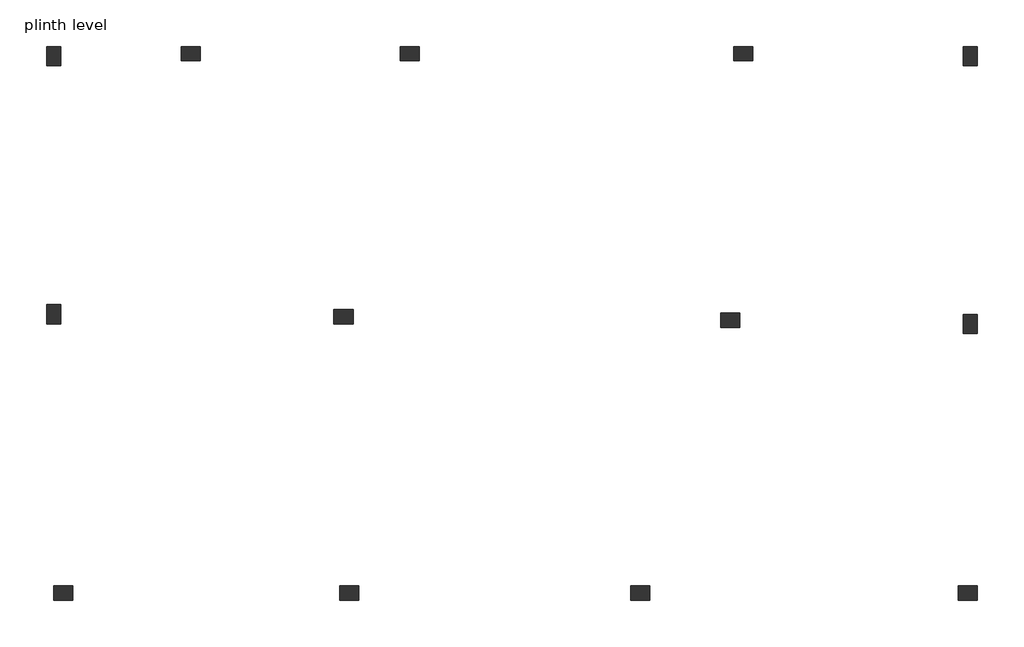
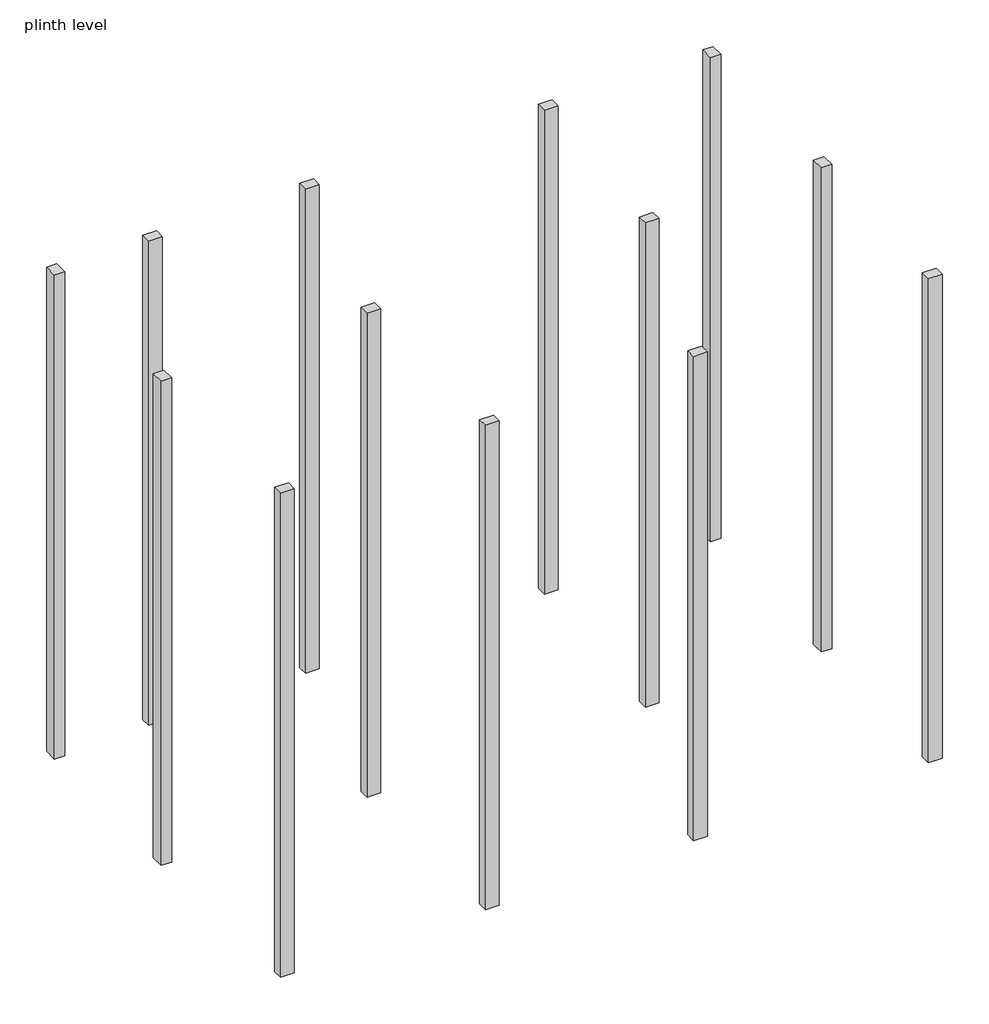
# One storey: 13 columns.
"""IFC4 building model written with IfcOpenShell, lengths in millimetres."""

from ifc_helpers import new_model, si_unit, frame, origin, place, context, project, spatial, polyline, outline, extrude, faceted_brep, element, save

model = new_model("IFC4")

# Units and contexts
model_context = context("Model", 3, world=origin())
ifc_project = project(units=[si_unit("LENGTHUNIT", "METRE", prefix="MILLI")], contexts=[model_context])

# Site, building, storey
site = spatial("IfcSite", under=ifc_project)
building = spatial("IfcBuilding", under=site)
storey = spatial("IfcBuildingStorey", under=building, Name="plinth level", Elevation=-1219.2)

# Columns
placement = place(None, origin())
element("IfcColumn", 1, ObjectType="Concrete-Rectangular-Column", at=placement, inside=storey, context=model_context, shape_type="SweptSolid", body=[
    extrude(outline(polyline([(-12643.368339, 9549.093496), (-12643.368339, 9244.293496), (-12871.968339, 9244.293496), (-12871.968339, 9549.093496), (-12643.368339, 9549.093496)])), frame((0.0, 0.0, -1219.2), z_axis=(0.0, 0.0, 1.0), x_axis=(1.0, 0.0, 0.0)), (0.0, 0.0, 1.0), 11430.0),
])
element("IfcColumn", 2, ObjectType="Concrete-Rectangular-Column", at=placement, inside=storey, context=model_context, shape_type="Brep", body=[
    faceted_brep([(-10719.318339, 9549.093496, -1219.2), (-10414.518339, 9549.093496, -1219.2), (-10414.518339, 9320.493496, -1219.2), (-10719.318339, 9320.493496, -1219.2), (-10719.318339, 9549.093496, 10210.8), (-10414.518339, 9549.093496, 10210.8), (-10414.518339, 9510.993496, 10210.8), (-10414.518339, 9320.493496, 10210.8), (-10414.518339, 9320.493496, 9906.0), (-10414.518339, 9320.493496, 7010.4), (-10414.518339, 9320.493496, 6705.6), (-10414.518339, 9320.493496, 3810.0), (-10414.518339, 9320.493496, 3505.2), (-10414.518339, 9320.493496, 609.6), (-10414.518339, 9320.493496, 304.8), (-10719.318339, 9320.493496, 10210.8), (-10719.318339, 9320.493496, 9906.0), (-10719.318339, 9320.493496, 7010.4), (-10719.318339, 9320.493496, 6705.6), (-10719.318339, 9320.493496, 3810.0), (-10719.318339, 9320.493496, 3505.2), (-10719.318339, 9320.493496, 609.6), (-10719.318339, 9320.493496, 304.8), (-10719.318339, 9510.993496, 10210.8)], [[[0, 1, 2, 3]], [[4, 5, 1, 0]], [[5, 6, 7, 8, 9, 10, 11, 12, 13, 14, 2, 1]], [[7, 15, 16, 17, 18, 19, 20, 21, 22, 3, 2, 14, 13, 12, 11, 10, 9, 8]], [[15, 23, 4, 0, 3, 22, 21, 20, 19, 18, 17, 16]], [[4, 23, 15, 7, 6, 5]]]),
])
element("IfcColumn", 3, ObjectType="Concrete-Rectangular-Column", at=placement, inside=storey, context=model_context, shape_type="Brep", body=[
    faceted_brep([(-7214.118339, 9549.093496, -1219.2), (-6909.318339, 9549.093496, -1219.2), (-6909.318339, 9320.493496, -1219.2), (-7214.118339, 9320.493496, -1219.2), (-7214.118339, 9549.093496, 10210.8), (-6909.318339, 9549.093496, 10210.8), (-6909.318339, 9510.993496, 10210.8), (-6909.318339, 9320.493496, 10210.8), (-6909.318339, 9320.493496, 9906.0), (-6909.318339, 9320.493496, 7010.4), (-6909.318339, 9320.493496, 6705.6), (-6909.318339, 9320.493496, 3810.0), (-6909.318339, 9320.493496, 3505.2), (-6909.318339, 9320.493496, 609.6), (-6909.318339, 9320.493496, 304.8), (-7214.118339, 9320.493496, 10210.8), (-7214.118339, 9320.493496, 9906.0), (-7214.118339, 9320.493496, 7010.4), (-7214.118339, 9320.493496, 6705.6), (-7214.118339, 9320.493496, 3810.0), (-7214.118339, 9320.493496, 3505.2), (-7214.118339, 9320.493496, 609.6), (-7214.118339, 9320.493496, 304.8), (-7214.118339, 9510.993496, 10210.8)], [[[0, 1, 2, 3]], [[4, 5, 1, 0]], [[5, 6, 7, 8, 9, 10, 11, 12, 13, 14, 2, 1]], [[7, 15, 16, 17, 18, 19, 20, 21, 22, 3, 2, 14, 13, 12, 11, 10, 9, 8]], [[15, 23, 4, 0, 3, 22, 21, 20, 19, 18, 17, 16]], [[4, 23, 15, 7, 6, 5]]]),
])
element("IfcColumn", 4, ObjectType="Concrete-Rectangular-Column", at=placement, inside=storey, context=model_context, shape_type="Brep", body=[
    faceted_brep([(-1880.118339, 9549.093496, -1219.2), (-1575.318339, 9549.093496, -1219.2), (-1575.318339, 9320.493496, -1219.2), (-1880.118339, 9320.493496, -1219.2), (-1880.118339, 9549.093496, 10210.8), (-1575.318339, 9549.093496, 10210.8), (-1575.318339, 9510.993496, 10210.8), (-1575.318339, 9320.493496, 10210.8), (-1575.318339, 9320.493496, 9906.0), (-1575.318339, 9320.493496, 7010.4), (-1575.318339, 9320.493496, 6705.6), (-1575.318339, 9320.493496, 3810.0), (-1575.318339, 9320.493496, 3505.2), (-1575.318339, 9320.493496, 609.6), (-1575.318339, 9320.493496, 304.8), (-1880.118339, 9320.493496, 10210.8), (-1880.118339, 9320.493496, 9906.0), (-1880.118339, 9320.493496, 7010.4), (-1880.118339, 9320.493496, 6705.6), (-1880.118339, 9320.493496, 3810.0), (-1880.118339, 9320.493496, 3505.2), (-1880.118339, 9320.493496, 609.6), (-1880.118339, 9320.493496, 304.8), (-1880.118339, 9510.993496, 10210.8)], [[[0, 1, 2, 3]], [[4, 5, 1, 0]], [[5, 6, 7, 8, 9, 10, 11, 12, 13, 14, 2, 1]], [[7, 15, 16, 17, 18, 19, 20, 21, 22, 3, 2, 14, 13, 12, 11, 10, 9, 8]], [[15, 23, 4, 0, 3, 22, 21, 20, 19, 18, 17, 16]], [[4, 23, 15, 7, 6, 5]]]),
])
element("IfcColumn", 5, ObjectType="Concrete-Rectangular-Column", at=placement, inside=storey, context=model_context, shape_type="SweptSolid", body=[
    extrude(outline(polyline([(1790.181661, 9244.293496), (1790.181661, 9549.093496), (2018.781661, 9549.093496), (2018.781661, 9244.293496), (1790.181661, 9244.293496)])), frame((0.0, 0.0, -1219.2), z_axis=(0.0, 0.0, 1.0), x_axis=(1.0, 0.0, 0.0)), (0.0, 0.0, 1.0), 11430.0),
])
element("IfcColumn", 6, ObjectType="Concrete-Rectangular-Column", at=placement, inside=storey, context=model_context, shape_type="Brep", body=[
    faceted_brep([(1790.181661, 4958.043496, -1219.2), (1790.181661, 5262.843496, -1219.2), (2018.781661, 5262.843496, -1219.2), (2018.781661, 4958.043496, -1219.2), (1790.181661, 4958.043496, 10210.8), (1790.181661, 5262.843496, 10210.8), (1790.181661, 5262.843496, 9906.0), (1790.181661, 5262.843496, 7010.4), (1790.181661, 5262.843496, 6705.6), (1790.181661, 5262.843496, 3810.0), (1790.181661, 5262.843496, 3505.2), (1790.181661, 5262.843496, 609.6), (1790.181661, 5262.843496, 304.8), (1790.181661, 4958.043496, 304.8), (1790.181661, 4958.043496, 609.6), (1790.181661, 4958.043496, 3505.2), (1790.181661, 4958.043496, 3810.0), (1790.181661, 4958.043496, 6705.6), (1790.181661, 4958.043496, 7010.4), (1790.181661, 4958.043496, 9906.0), (2018.781661, 5262.843496, 10210.8), (2018.781661, 5262.843496, 9906.0), (2018.781661, 5262.843496, 7010.4), (2018.781661, 5262.843496, 6705.6), (2018.781661, 5262.843496, 3810.0), (2018.781661, 5262.843496, 3505.2), (2018.781661, 5262.843496, 609.6), (2018.781661, 5262.843496, 304.8), (2018.781661, 4958.043496, 10210.8), (2018.781661, 4958.043496, 9906.0), (2018.781661, 4958.043496, 7010.4), (2018.781661, 4958.043496, 6705.6), (2018.781661, 4958.043496, 3810.0), (2018.781661, 4958.043496, 3505.2), (2018.781661, 4958.043496, 609.6), (2018.781661, 4958.043496, 304.8)], [[[0, 1, 2, 3]], [[4, 5, 6, 7, 8, 9, 10, 11, 12, 1, 0, 13, 14, 15, 16, 17, 18, 19]], [[5, 20, 21, 22, 23, 24, 25, 26, 27, 2, 1, 12, 11, 10, 9, 8, 7, 6]], [[20, 28, 29, 30, 31, 32, 33, 34, 35, 3, 2, 27, 26, 25, 24, 23, 22, 21]], [[28, 4, 19, 18, 17, 16, 15, 14, 13, 0, 3, 35, 34, 33, 32, 31, 30, 29]], [[4, 28, 20, 5]]]),
])
element("IfcColumn", 7, ObjectType="Concrete-Rectangular-Column", at=placement, inside=storey, context=model_context, shape_type="Brep", body=[
    faceted_brep([(-1784.868339, 5053.293496, -1219.2), (-2089.668339, 5053.293496, -1219.2), (-2089.668339, 5281.893496, -1219.2), (-1784.868339, 5281.893496, -1219.2), (-1784.868339, 5053.293496, 10210.8), (-1842.018339, 5053.293496, 10210.8), (-2089.668339, 5053.293496, 10210.8), (-2089.668339, 5053.293496, 9906.0), (-2089.668339, 5053.293496, 7010.4), (-2089.668339, 5053.293496, 6705.6), (-2089.668339, 5053.293496, 3810.0), (-2089.668339, 5053.293496, 3505.2), (-2089.668339, 5053.293496, 609.6), (-2089.668339, 5053.293496, 304.8), (-1784.868339, 5053.293496, 304.8), (-1784.868339, 5053.293496, 609.6), (-1784.868339, 5053.293496, 3505.2), (-1784.868339, 5053.293496, 3810.0), (-1784.868339, 5053.293496, 6705.6), (-1784.868339, 5053.293496, 7010.4), (-1784.868339, 5053.293496, 9906.0), (-2089.668339, 5224.743496, 10210.8), (-2089.668339, 5281.893496, 10210.8), (-1842.018339, 5281.893496, 10210.8), (-1784.868339, 5281.893496, 10210.8), (-1784.868339, 5281.893496, 9906.0), (-1784.868339, 5281.893496, 7010.4), (-1784.868339, 5281.893496, 6705.6), (-1784.868339, 5281.893496, 3810.0), (-1784.868339, 5281.893496, 3505.2), (-1784.868339, 5281.893496, 609.6), (-1784.868339, 5281.893496, 304.8)], [[[0, 1, 2, 3]], [[4, 5, 6, 7, 8, 9, 10, 11, 12, 13, 1, 0, 14, 15, 16, 17, 18, 19, 20]], [[6, 21, 22, 2, 1, 13, 12, 11, 10, 9, 8, 7]], [[22, 23, 24, 25, 26, 27, 28, 29, 30, 31, 3, 2]], [[24, 4, 20, 19, 18, 17, 16, 15, 14, 0, 3, 31, 30, 29, 28, 27, 26, 25]], [[4, 24, 23, 22, 21, 6, 5]]]),
])
element("IfcColumn", 8, ObjectType="Concrete-Rectangular-Column", at=placement, inside=storey, context=model_context, shape_type="SweptSolid", body=[
    extrude(outline(polyline([(-7969.768339, 5110.443496), (-8274.568339, 5110.443496), (-8274.568339, 5339.043496), (-7969.768339, 5339.043496), (-7969.768339, 5110.443496)])), frame((0.0, 0.0, -1219.2), z_axis=(0.0, 0.0, 1.0), x_axis=(1.0, 0.0, 0.0)), (0.0, 0.0, 1.0), 11430.0),
])
element("IfcColumn", 9, ObjectType="Concrete-Rectangular-Column", at=placement, inside=storey, context=model_context, shape_type="SweptSolid", body=[
    extrude(outline(polyline([(-12643.368339, 5415.243496), (-12643.368339, 5110.443496), (-12871.968339, 5110.443496), (-12871.968339, 5415.243496), (-12643.368339, 5415.243496)])), frame((0.0, 0.0, -1219.2), z_axis=(0.0, 0.0, 1.0), x_axis=(1.0, 0.0, 0.0)), (0.0, 0.0, 1.0), 11430.0),
])
element("IfcColumn", 10, ObjectType="Concrete-Rectangular-Column", at=placement, inside=storey, context=model_context, shape_type="SweptSolid", body=[
    extrude(outline(polyline([(-12757.668339, 913.093496), (-12452.868339, 913.093496), (-12452.868339, 684.493496), (-12757.668339, 684.493496), (-12757.668339, 913.093496)])), frame((0.0, 0.0, -1219.2), z_axis=(0.0, 0.0, 1.0), x_axis=(1.0, 0.0, 0.0)), (0.0, 0.0, 1.0), 11430.0),
])
element("IfcColumn", 11, ObjectType="Concrete-Rectangular-Column", at=placement, inside=storey, context=model_context, shape_type="Brep", body=[
    faceted_brep([(-8179.318339, 913.093496, -1219.2), (-7874.518339, 913.093496, -1219.2), (-7874.518339, 684.493496, -1219.2), (-8179.318339, 684.493496, -1219.2), (-8179.318339, 913.093496, 10210.8), (-7874.518339, 913.093496, 10210.8), (-7874.518339, 913.093496, 9906.0), (-7874.518339, 913.093496, 7010.4), (-7874.518339, 913.093496, 6705.6), (-7874.518339, 913.093496, 3810.0), (-7874.518339, 913.093496, 3505.2), (-7874.518339, 913.093496, 609.6), (-7874.518339, 913.093496, 304.8), (-8179.318339, 913.093496, 304.8), (-8179.318339, 913.093496, 609.6), (-8179.318339, 913.093496, 3505.2), (-8179.318339, 913.093496, 3810.0), (-8179.318339, 913.093496, 6705.6), (-8179.318339, 913.093496, 7010.4), (-8179.318339, 913.093496, 9906.0), (-7874.518339, 684.493496, 10210.8), (-7874.518339, 684.493496, 9906.0), (-7874.518339, 684.493496, 7010.4), (-7874.518339, 684.493496, 6705.6), (-7874.518339, 684.493496, 3810.0), (-7874.518339, 684.493496, 3505.2), (-7874.518339, 684.493496, 609.6), (-7874.518339, 684.493496, 304.8), (-8179.318339, 684.493496, 10210.8), (-8179.318339, 684.493496, 9906.0), (-8179.318339, 684.493496, 7010.4), (-8179.318339, 684.493496, 6705.6), (-8179.318339, 684.493496, 3810.0), (-8179.318339, 684.493496, 3505.2), (-8179.318339, 684.493496, 609.6), (-8179.318339, 684.493496, 304.8)], [[[0, 1, 2, 3]], [[4, 5, 6, 7, 8, 9, 10, 11, 12, 1, 0, 13, 14, 15, 16, 17, 18, 19]], [[5, 20, 21, 22, 23, 24, 25, 26, 27, 2, 1, 12, 11, 10, 9, 8, 7, 6]], [[20, 28, 29, 30, 31, 32, 33, 34, 35, 3, 2, 27, 26, 25, 24, 23, 22, 21]], [[28, 4, 19, 18, 17, 16, 15, 14, 13, 0, 3, 35, 34, 33, 32, 31, 30, 29]], [[4, 28, 20, 5]]]),
])
element("IfcColumn", 12, ObjectType="Concrete-Rectangular-Column", at=placement, inside=storey, context=model_context, shape_type="Brep", body=[
    faceted_brep([(-3531.016739, 913.093496, -1219.2), (-3226.216739, 913.093496, -1219.2), (-3226.216739, 684.493496, -1219.2), (-3531.016739, 684.493496, -1219.2), (-3531.016739, 913.093496, 10210.8), (-3226.216739, 913.093496, 10210.8), (-3226.216739, 913.093496, 9906.0), (-3226.216739, 913.093496, 7010.4), (-3226.216739, 913.093496, 6705.6), (-3226.216739, 913.093496, 3810.0), (-3226.216739, 913.093496, 3505.2), (-3226.216739, 913.093496, 609.6), (-3226.216739, 913.093496, 304.8), (-3531.016739, 913.093496, 304.8), (-3531.016739, 913.093496, 609.6), (-3531.016739, 913.093496, 3505.2), (-3531.016739, 913.093496, 3810.0), (-3531.016739, 913.093496, 6705.6), (-3531.016739, 913.093496, 7010.4), (-3531.016739, 913.093496, 9906.0), (-3226.216739, 684.493496, 10210.8), (-3226.216739, 684.493496, 9906.0), (-3226.216739, 684.493496, 7010.4), (-3226.216739, 684.493496, 6705.6), (-3226.216739, 684.493496, 3810.0), (-3226.216739, 684.493496, 3505.2), (-3226.216739, 684.493496, 609.6), (-3226.216739, 684.493496, 304.8), (-3531.016739, 684.493496, 10210.8), (-3531.016739, 684.493496, 9906.0), (-3531.016739, 684.493496, 7010.4), (-3531.016739, 684.493496, 6705.6), (-3531.016739, 684.493496, 3810.0), (-3531.016739, 684.493496, 3505.2), (-3531.016739, 684.493496, 609.6), (-3531.016739, 684.493496, 304.8)], [[[0, 1, 2, 3]], [[4, 5, 6, 7, 8, 9, 10, 11, 12, 1, 0, 13, 14, 15, 16, 17, 18, 19]], [[5, 20, 21, 22, 23, 24, 25, 26, 27, 2, 1, 12, 11, 10, 9, 8, 7, 6]], [[20, 28, 29, 30, 31, 32, 33, 34, 35, 3, 2, 27, 26, 25, 24, 23, 22, 21]], [[28, 4, 19, 18, 17, 16, 15, 14, 13, 0, 3, 35, 34, 33, 32, 31, 30, 29]], [[4, 28, 20, 5]]]),
])
element("IfcColumn", 13, ObjectType="Concrete-Rectangular-Column", at=placement, inside=storey, context=model_context, shape_type="SweptSolid", body=[
    extrude(outline(polyline([(1713.981661, 913.093496), (2018.781661, 913.093496), (2018.781661, 684.493496), (1713.981661, 684.493496), (1713.981661, 913.093496)])), frame((0.0, 0.0, -1219.2), z_axis=(0.0, 0.0, 1.0), x_axis=(1.0, 0.0, 0.0)), (0.0, 0.0, 1.0), 11430.0),
])

save(model, "model.ifc")

# Revit data of these elements
# Type "Concrete-Rectangular-Column"
#   Assembly Code = "B10"
#   b = 0.75 ft
#   h = 1 ft
#   Structural Material [instance default] = Concrete, Cast-in-Place gray
# Elements 1, 2, 3, 4, 5, 6, 7, 8, 9, 10, 11, 12, 13 (IfcColumn, "Concrete-Rectangular-Column")
#   Structural Material = Concrete, Cast-in-Place gray
#   Phase Created = New Construction
#   Materials on its faces: "Concrete, Cast-in-Place gray"
# Materials
#   "Concrete, Cast-in-Place gray": class "Concrete", colour RGB 192 192 192, transparency 0, Description = "Cast-in-place concrete", Cost = 0
